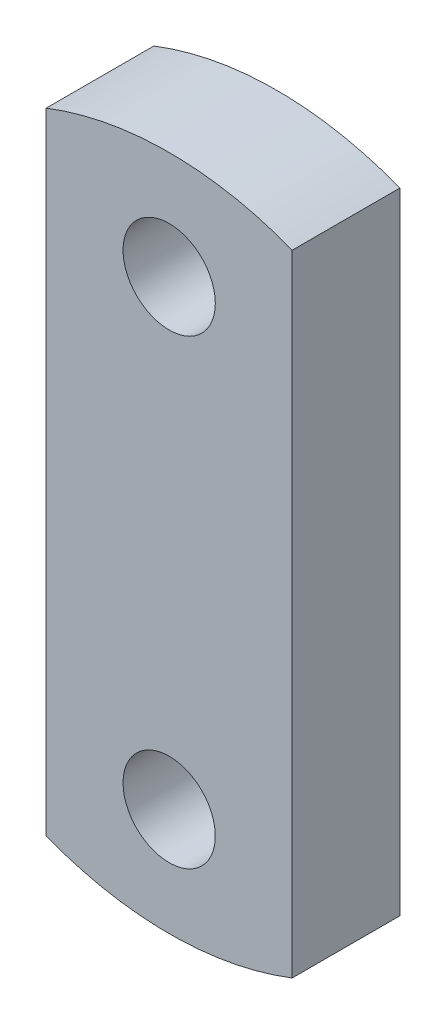
SolidWorks part; units mm, degrees
material "Alloy Steel"
ref_plane "Front Plane" through (0, 0, 0) normal (0, 0, 1) x (1, 0, 0)
ref_plane "Top Plane" through (0, 0, 0) normal (0, 1, 0) x (1, 0, 0)
ref_plane "Right Plane" through (0, 0, 0) normal (1, 0, 0) x (0, 0, -1)
sketch "Plate Profile with Bores" plane through (0, 0, 0) normal (0, 0, 1) x (1, 0, 0)
  line L0 (0, 0) -> (-191.827, 0) construction
  line L2 (-40, -102.4695) -> (-40, 102.4695)
  line L4 (40, -102.4695) -> (40, 102.4695)
  line L5 (-40, -102.4695) -> (40, 102.4695) construction
  line L6 (-40, 102.4695) -> (40, -102.4695) construction
  arc A0 (-40, 102.4695) -> (40, 102.4695) centre (0, 0) cw
  arc A1 (-40, -102.4695) -> (40, -102.4695) centre (0, 0) ccw
  circle A2 centre (0, 75) radius 15
  circle A3 centre (0, -75) radius 15
  point P0 (0, 0)
  point P10 (0, 110)
  point P11 (0, -110)
  dimension "D1" = 110
  dimension "D4" = 30
  dimension "D2" = 80
  dimension "D3" = 220
  dimension "D5" = 75
extrude "Crosshead Plate 35mm" add sketch "Plate Profile with Bores" along normal mid plane 35
